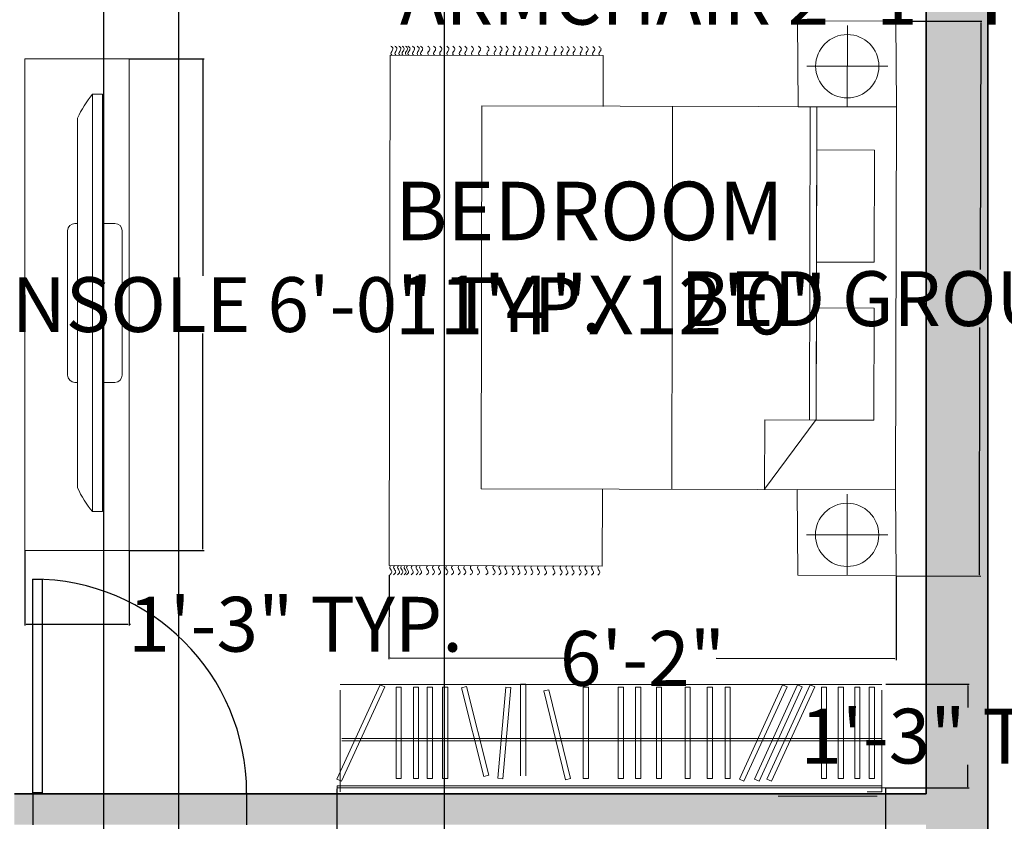
# Model space of a CAD drawing. Units: inches. Extents: x -4737294 to -4736756, y 1716389 to 1717040.
# Tile 23 of 25: x -4736996 to -4736853, y 1716845 to 1716962. Entities that reach past the tile are written whole.
import ezdxf

# ---------------------------------------------------------------- set-up
doc = ezdxf.new("R2010")
doc.units = ezdxf.units.IN
doc.header["$MEASUREMENT"] = 0
for name, color, linetype, lineweight in [('A-ANNO-DIMS', 2, 'Continuous', 18), ('A-AREA-IDEN', 250, 'Continuous', 18), ('A-WALL-PATT', 244, 'Continuous', 13), ('closet', 252, 'Continuous', 18), ('doors', 252, 'Continuous', 25), ('furniture', 250, 'Continuous', 18), ('walls', 252, 'Continuous', 35)]:
    doc.layers.add(name, color=color, linetype=linetype, lineweight=lineweight)
doc.styles.get("Standard").update_dxf_attribs({"font": 'arial.ttf'})
doc.dimstyles.get("Standard").update_dxf_attribs({"dimtxt": 8, "dimasz": 0.18, "dimexe": 0.18, "dimexo": 0.0625, "dimgap": 0.09, "dimtad": 0, "dimtih": 1, "dimtoh": 1, "dimzin": 0, "dimdsep": 46, "dimlunit": 3, "dimtxsty": 'Standard', "dimcen": 0.09, "dimadec": 0, "dimazin": 0, "dimtfac": 1, "dimtofl": 0, "dimtmove": 0, "dimatfit": 3, "dimfxl": 1, "dimtolj": 1, "dimtzin": 0, "dimarcsym": 0})

# ---------------------------------------------------------------- blocks, each defined once
blk = doc.blocks.new('*D22')
at = {"layer": 'A-ANNO-DIMS', "color": 0, "lineweight": -2, "transparency": 16777216}
for p, q in [((-4736855.08, 1717002.06), (-4736830.06, 1717002.06)), ((-4736830.24, 1717001.88), (-4736830.24, 1716736.22)), ((-4736830.24, 1716462.24), (-4736830.24, 1716727.91)), ((-4736855.08, 1716462.06), (-4736830.06, 1716462.06))]:
    blk.add_line(p, q, dxfattribs=at)
at = {"layer": 'A-ANNO-DIMS', "color": 0, "transparency": 16777216}
for points in [[(-4736830.27, 1717001.88), (-4736830.21, 1717001.88), (-4736830.24, 1717002.06)], [(-4736830.27, 1716462.24), (-4736830.21, 1716462.24), (-4736830.24, 1716462.06)]]:
    blk.add_solid(points, dxfattribs=at)
at = {"layer": 'Defpoints', "color": 0, "transparency": 16777216}
for p in [(-4736855.14, 1717002.06), (-4736830.24, 1717002.06), (-4736855.14, 1716462.06)]:
    blk.add_point(p, dxfattribs=at)
at = {"layer": 'A-ANNO-DIMS', "color": 0, "transparency": 16777216, "insert": (-4736830.24, 1716732.06), "char_height": 8, "attachment_point": 5}
blk.add_mtext("\\A1;45'", dxfattribs=at)
blk = doc.blocks.new('CARPET')
at = {"layer": 'furniture'}
for p, q in [((-51.53, -98.11), (-51.53, -55.12)), ((-51.53, -55.12), (-41.27, -55.12)), ((36, -55.12), (51.55, -55.12)), ((51.55, -55.12), (51.55, -98.11)), ((51.55, -98.11), (-51.53, -98.11))]:
    blk.add_line(p, q, dxfattribs=at)
for points, knots in [([(-53.37, -55.99), (-53.22, -55.8), (-52.9, -55.41), (-52.34, -55.8), (-51.89, -56.08), (-51.65, -55.91), (-51.53, -55.83)], [0, 0, 0, 0, 0.653278, 1.290138, 1.740457, 2.114451, 2.114451, 2.114451, 2.114451]), ([(53.37, -55.99), (53.22, -55.8), (52.9, -55.41), (52.34, -55.8), (51.89, -56.08), (51.65, -55.91), (51.53, -55.83)], [0, 0, 0, 0, 0.653278, 1.290138, 1.740457, 2.114451, 2.114451, 2.114451, 2.114451]), ([(-53.37, -57.26), (-53.22, -57.07), (-52.9, -56.67), (-52.34, -57.07), (-51.89, -57.35), (-51.65, -57.17), (-51.53, -57.1)], [0, 0, 0, 0, 0.653278, 1.290138, 1.740457, 2.114451, 2.114451, 2.114451, 2.114451]), ([(53.37, -57.26), (53.22, -57.07), (52.9, -56.67), (52.34, -57.07), (51.89, -57.35), (51.65, -57.17), (51.53, -57.1)], [0, 0, 0, 0, 0.653278, 1.290138, 1.740457, 2.114451, 2.114451, 2.114451, 2.114451]), ([(-53.37, -58.59), (-53.22, -58.4), (-52.9, -58.01), (-52.34, -58.4), (-51.89, -58.68), (-51.65, -58.5), (-51.53, -58.43)], [0, 0, 0, 0, 0.653278, 1.290138, 1.740457, 2.114451, 2.114451, 2.114451, 2.114451]), ([(-53.37, -59.78), (-53.22, -59.58), (-52.9, -59.19), (-52.34, -59.58), (-51.89, -59.86), (-51.65, -59.69), (-51.53, -59.61)], [0, 0, 0, 0, 0.653278, 1.290138, 1.740457, 2.114451, 2.114451, 2.114451, 2.114451]), ([(53.37, -58.59), (53.22, -58.4), (52.9, -58.01), (52.34, -58.4), (51.89, -58.68), (51.65, -58.5), (51.53, -58.43)], [0, 0, 0, 0, 0.653278, 1.290138, 1.740457, 2.114451, 2.114451, 2.114451, 2.114451]), ([(53.37, -59.78), (53.22, -59.58), (52.9, -59.19), (52.34, -59.58), (51.89, -59.86), (51.65, -59.69), (51.53, -59.61)], [0, 0, 0, 0, 0.653278, 1.290138, 1.740457, 2.114451, 2.114451, 2.114451, 2.114451]), ([(-53.37, -61.22), (-53.22, -61.02), (-52.9, -60.63), (-52.34, -61.02), (-51.89, -61.3), (-51.65, -61.13), (-51.53, -61.05)], [0, 0, 0, 0, 0.653278, 1.290138, 1.740457, 2.114451, 2.114451, 2.114451, 2.114451]), ([(53.37, -61.22), (53.22, -61.02), (52.9, -60.63), (52.34, -61.02), (51.89, -61.3), (51.65, -61.13), (51.53, -61.05)], [0, 0, 0, 0, 0.653278, 1.290138, 1.740457, 2.114451, 2.114451, 2.114451, 2.114451]), ([(-53.37, -62.44), (-53.22, -62.25), (-52.9, -61.86), (-52.34, -62.25), (-51.89, -62.53), (-51.65, -62.36), (-51.53, -62.28)], [0, 0, 0, 0, 0.653278, 1.290138, 1.740457, 2.114451, 2.114451, 2.114451, 2.114451]), ([(-53.37, -63.63), (-53.22, -63.43), (-52.9, -63.04), (-52.34, -63.43), (-51.89, -63.72), (-51.65, -63.54), (-51.53, -63.46)], [0, 0, 0, 0, 0.653278, 1.290138, 1.740457, 2.114451, 2.114451, 2.114451, 2.114451]), ([(53.37, -62.44), (53.22, -62.25), (52.9, -61.86), (52.34, -62.25), (51.89, -62.53), (51.65, -62.36), (51.53, -62.28)], [0, 0, 0, 0, 0.653278, 1.290138, 1.740457, 2.114451, 2.114451, 2.114451, 2.114451]), ([(53.37, -63.63), (53.22, -63.43), (52.9, -63.04), (52.34, -63.43), (51.89, -63.72), (51.65, -63.54), (51.53, -63.46)], [0, 0, 0, 0, 0.653278, 1.290138, 1.740457, 2.114451, 2.114451, 2.114451, 2.114451]), ([(-53.37, -65.07), (-53.22, -64.87), (-52.9, -64.48), (-52.34, -64.87), (-51.89, -65.15), (-51.65, -64.98), (-51.53, -64.9)], [0, 0, 0, 0, 0.653278, 1.290138, 1.740457, 2.114451, 2.114451, 2.114451, 2.114451]), ([(53.37, -65.07), (53.22, -64.87), (52.9, -64.48), (52.34, -64.87), (51.89, -65.15), (51.65, -64.98), (51.53, -64.9)], [0, 0, 0, 0, 0.653278, 1.290138, 1.740457, 2.114451, 2.114451, 2.114451, 2.114451]), ([(-53.37, -66.76), (-53.22, -66.56), (-52.9, -66.17), (-52.34, -66.56), (-51.89, -66.84), (-51.65, -66.67), (-51.53, -66.59)], [0, 0, 0, 0, 0.653278, 1.290138, 1.740457, 2.114451, 2.114451, 2.114451, 2.114451]), ([(53.37, -66.76), (53.22, -66.56), (52.9, -66.17), (52.34, -66.56), (51.89, -66.84), (51.65, -66.67), (51.53, -66.59)], [0, 0, 0, 0, 0.653278, 1.290138, 1.740457, 2.114451, 2.114451, 2.114451, 2.114451]), ([(-53.37, -68.2), (-53.22, -68), (-52.9, -67.61), (-52.34, -68), (-51.89, -68.28), (-51.65, -68.11), (-51.53, -68.03)], [0, 0, 0, 0, 0.653278, 1.290138, 1.740457, 2.114451, 2.114451, 2.114451, 2.114451]), ([(-53.37, -69.53), (-53.22, -69.33), (-52.9, -68.94), (-52.34, -69.33), (-51.89, -69.61), (-51.65, -69.44), (-51.53, -69.36)], [0, 0, 0, 0, 0.653278, 1.290138, 1.740457, 2.114451, 2.114451, 2.114451, 2.114451]), ([(53.37, -68.2), (53.22, -68), (52.9, -67.61), (52.34, -68), (51.89, -68.28), (51.65, -68.11), (51.53, -68.03)], [0, 0, 0, 0, 0.653278, 1.290138, 1.740457, 2.114451, 2.114451, 2.114451, 2.114451]), ([(53.37, -69.53), (53.22, -69.33), (52.9, -68.94), (52.34, -69.33), (51.89, -69.61), (51.65, -69.44), (51.53, -69.36)], [0, 0, 0, 0, 0.653278, 1.290138, 1.740457, 2.114451, 2.114451, 2.114451, 2.114451]), ([(-53.37, -70.79), (-53.22, -70.6), (-52.9, -70.21), (-52.34, -70.6), (-51.89, -70.88), (-51.65, -70.7), (-51.53, -70.63)], [0, 0, 0, 0, 0.653278, 1.290138, 1.740457, 2.114451, 2.114451, 2.114451, 2.114451]), ([(53.37, -70.79), (53.22, -70.6), (52.9, -70.21), (52.34, -70.6), (51.89, -70.88), (51.65, -70.7), (51.53, -70.63)], [0, 0, 0, 0, 0.653278, 1.290138, 1.740457, 2.114451, 2.114451, 2.114451, 2.114451]), ([(-53.37, -72.12), (-53.22, -71.93), (-52.9, -71.54), (-52.34, -71.93), (-51.89, -72.21), (-51.65, -72.04), (-51.53, -71.96)], [0, 0, 0, 0, 0.653278, 1.290138, 1.740457, 2.114451, 2.114451, 2.114451, 2.114451]), ([(-53.37, -73.31), (-53.22, -73.11), (-52.9, -72.72), (-52.34, -73.11), (-51.89, -73.4), (-51.65, -73.22), (-51.53, -73.14)], [0, 0, 0, 0, 0.653278, 1.290138, 1.740457, 2.114451, 2.114451, 2.114451, 2.114451]), ([(53.37, -72.12), (53.22, -71.93), (52.9, -71.54), (52.34, -71.93), (51.89, -72.21), (51.65, -72.04), (51.53, -71.96)], [0, 0, 0, 0, 0.653278, 1.290138, 1.740457, 2.114451, 2.114451, 2.114451, 2.114451]), ([(53.37, -73.31), (53.22, -73.11), (52.9, -72.72), (52.34, -73.11), (51.89, -73.4), (51.65, -73.22), (51.53, -73.14)], [0, 0, 0, 0, 0.653278, 1.290138, 1.740457, 2.114451, 2.114451, 2.114451, 2.114451]), ([(-53.37, -74.75), (-53.22, -74.55), (-52.9, -74.16), (-52.34, -74.55), (-51.89, -74.83), (-51.65, -74.66), (-51.53, -74.58)], [0, 0, 0, 0, 0.653278, 1.290138, 1.740457, 2.114451, 2.114451, 2.114451, 2.114451]), ([(53.37, -74.75), (53.22, -74.55), (52.9, -74.16), (52.34, -74.55), (51.89, -74.83), (51.65, -74.66), (51.53, -74.58)], [0, 0, 0, 0, 0.653278, 1.290138, 1.740457, 2.114451, 2.114451, 2.114451, 2.114451]), ([(-53.37, -75.98), (-53.22, -75.78), (-52.9, -75.39), (-52.34, -75.78), (-51.89, -76.06), (-51.65, -75.89), (-51.53, -75.81)], [0, 0, 0, 0, 0.653278, 1.290138, 1.740457, 2.114451, 2.114451, 2.114451, 2.114451]), ([(-53.37, -77.16), (-53.22, -76.96), (-52.9, -76.57), (-52.34, -76.96), (-51.89, -77.25), (-51.65, -77.07), (-51.53, -76.99)], [0, 0, 0, 0, 0.653278, 1.290138, 1.740457, 2.114451, 2.114451, 2.114451, 2.114451]), ([(53.37, -75.98), (53.22, -75.78), (52.9, -75.39), (52.34, -75.78), (51.89, -76.06), (51.65, -75.89), (51.53, -75.81)], [0, 0, 0, 0, 0.653278, 1.290138, 1.740457, 2.114451, 2.114451, 2.114451, 2.114451]), ([(53.37, -77.16), (53.22, -76.96), (52.9, -76.57), (52.34, -76.96), (51.89, -77.25), (51.65, -77.07), (51.53, -76.99)], [0, 0, 0, 0, 0.653278, 1.290138, 1.740457, 2.114451, 2.114451, 2.114451, 2.114451]), ([(-53.37, -78.6), (-53.22, -78.4), (-52.9, -78.01), (-52.34, -78.4), (-51.89, -78.68), (-51.65, -78.51), (-51.53, -78.43)], [0, 0, 0, 0, 0.653278, 1.290138, 1.740457, 2.114451, 2.114451, 2.114451, 2.114451]), ([(53.37, -78.6), (53.22, -78.4), (52.9, -78.01), (52.34, -78.4), (51.89, -78.68), (51.65, -78.51), (51.53, -78.43)], [0, 0, 0, 0, 0.653278, 1.290138, 1.740457, 2.114451, 2.114451, 2.114451, 2.114451]), ([(-53.37, -80.29), (-53.22, -80.09), (-52.9, -79.7), (-52.34, -80.09), (-51.89, -80.37), (-51.65, -80.2), (-51.53, -80.12)], [0, 0, 0, 0, 0.653278, 1.290138, 1.740457, 2.114451, 2.114451, 2.114451, 2.114451]), ([(-53.37, -81.73), (-53.22, -81.53), (-52.9, -81.14), (-52.34, -81.53), (-51.89, -81.81), (-51.65, -81.64), (-51.53, -81.56)], [0, 0, 0, 0, 0.653278, 1.290138, 1.740457, 2.114451, 2.114451, 2.114451, 2.114451]), ([(53.37, -80.29), (53.22, -80.09), (52.9, -79.7), (52.34, -80.09), (51.89, -80.37), (51.65, -80.2), (51.53, -80.12)], [0, 0, 0, 0, 0.653278, 1.290138, 1.740457, 2.114451, 2.114451, 2.114451, 2.114451]), ([(53.37, -81.73), (53.22, -81.53), (52.9, -81.14), (52.34, -81.53), (51.89, -81.81), (51.65, -81.64), (51.53, -81.56)], [0, 0, 0, 0, 0.653278, 1.290138, 1.740457, 2.114451, 2.114451, 2.114451, 2.114451]), ([(-53.37, -83.06), (-53.22, -82.86), (-52.9, -82.47), (-52.34, -82.86), (-51.89, -83.14), (-51.65, -82.97), (-51.53, -82.89)], [0, 0, 0, 0, 0.653278, 1.290138, 1.740457, 2.114451, 2.114451, 2.114451, 2.114451]), ([(53.37, -83.06), (53.22, -82.86), (52.9, -82.47), (52.34, -82.86), (51.89, -83.14), (51.65, -82.97), (51.53, -82.89)], [0, 0, 0, 0, 0.653278, 1.290138, 1.740457, 2.114451, 2.114451, 2.114451, 2.114451]), ([(-53.37, -84.18), (-53.22, -83.99), (-52.9, -83.6), (-52.34, -83.99), (-51.89, -84.27), (-51.65, -84.09), (-51.53, -84.02)], [0, 0, 0, 0, 0.653278, 1.290138, 1.740457, 2.114451, 2.114451, 2.114451, 2.114451]), ([(-53.37, -85.51), (-53.22, -85.32), (-52.9, -84.93), (-52.34, -85.32), (-51.89, -85.6), (-51.65, -85.42), (-51.53, -85.35)], [0, 0, 0, 0, 0.653278, 1.290138, 1.740457, 2.114451, 2.114451, 2.114451, 2.114451]), ([(53.37, -84.18), (53.22, -83.99), (52.9, -83.6), (52.34, -83.99), (51.89, -84.27), (51.65, -84.09), (51.53, -84.02)], [0, 0, 0, 0, 0.653278, 1.290138, 1.740457, 2.114451, 2.114451, 2.114451, 2.114451]), ([(53.37, -85.51), (53.22, -85.32), (52.9, -84.93), (52.34, -85.32), (51.89, -85.6), (51.65, -85.42), (51.53, -85.35)], [0, 0, 0, 0, 0.653278, 1.290138, 1.740457, 2.114451, 2.114451, 2.114451, 2.114451]), ([(-53.37, -86.7), (-53.22, -86.5), (-52.9, -86.11), (-52.34, -86.5), (-51.89, -86.78), (-51.65, -86.61), (-51.53, -86.53)], [0, 0, 0, 0, 0.653278, 1.290138, 1.740457, 2.114451, 2.114451, 2.114451, 2.114451]), ([(53.37, -86.7), (53.22, -86.5), (52.9, -86.11), (52.34, -86.5), (51.89, -86.78), (51.65, -86.61), (51.53, -86.53)], [0, 0, 0, 0, 0.653278, 1.290138, 1.740457, 2.114451, 2.114451, 2.114451, 2.114451]), ([(-53.37, -88.14), (-53.22, -87.94), (-52.9, -87.55), (-52.34, -87.94), (-51.89, -88.22), (-51.65, -88.05), (-51.53, -87.97)], [0, 0, 0, 0, 0.653278, 1.290138, 1.740457, 2.114451, 2.114451, 2.114451, 2.114451]), ([(-53.37, -89.36), (-53.22, -89.17), (-52.9, -88.78), (-52.34, -89.17), (-51.89, -89.45), (-51.65, -89.28), (-51.53, -89.2)], [0, 0, 0, 0, 0.653278, 1.290138, 1.740457, 2.114451, 2.114451, 2.114451, 2.114451]), ([(53.37, -88.14), (53.22, -87.94), (52.9, -87.55), (52.34, -87.94), (51.89, -88.22), (51.65, -88.05), (51.53, -87.97)], [0, 0, 0, 0, 0.653278, 1.290138, 1.740457, 2.114451, 2.114451, 2.114451, 2.114451]), ([(53.37, -89.36), (53.22, -89.17), (52.9, -88.78), (52.34, -89.17), (51.89, -89.45), (51.65, -89.28), (51.53, -89.2)], [0, 0, 0, 0, 0.653278, 1.290138, 1.740457, 2.114451, 2.114451, 2.114451, 2.114451]), ([(-53.37, -90.55), (-53.22, -90.35), (-52.9, -89.96), (-52.34, -90.35), (-51.89, -90.64), (-51.65, -90.46), (-51.53, -90.38)], [0, 0, 0, 0, 0.653278, 1.290138, 1.740457, 2.114451, 2.114451, 2.114451, 2.114451]), ([(53.37, -90.55), (53.22, -90.35), (52.9, -89.96), (52.34, -90.35), (51.9, -90.63), (51.66, -90.47), (51.55, -90.4)], [0, 0, 0, 0, 0.653278, 1.290138, 1.740457, 2.0926, 2.0926, 2.0926, 2.0926]), ([(-53.37, -91.99), (-53.22, -91.79), (-52.9, -91.4), (-52.34, -91.79), (-51.89, -92.07), (-51.65, -91.9), (-51.53, -91.82)], [0, 0, 0, 0, 0.653278, 1.290138, 1.740457, 2.114451, 2.114451, 2.114451, 2.114451]), ([(-53.37, -92.69), (-53.22, -92.48), (-52.9, -92.08), (-52.35, -92.49), (-51.89, -92.77), (-51.65, -92.6), (-51.53, -92.52)], [0, 0, 0, 0, 0.663904, 1.307406, 1.757725, 2.131719, 2.131719, 2.131719, 2.131719]), ([(-53.37, -93.61), (-53.22, -93.42), (-52.9, -93.03), (-52.34, -93.42), (-51.89, -93.7), (-51.65, -93.52), (-51.53, -93.45)], [0, 0, 0, 0, 0.653278, 1.290138, 1.740457, 2.114451, 2.114451, 2.114451, 2.114451]), ([(53.37, -91.99), (53.22, -91.79), (52.9, -91.4), (52.34, -91.79), (51.9, -92.07), (51.66, -91.91), (51.55, -91.83)], [0, 0, 0, 0, 0.653278, 1.290138, 1.740457, 2.0926, 2.0926, 2.0926, 2.0926]), ([(53.37, -92.69), (53.22, -92.49), (52.9, -92.09), (52.34, -92.49), (51.9, -92.77), (51.66, -92.61), (51.55, -92.53)], [0, 0, 0, 0, 0.656792, 1.295826, 1.746145, 2.098292, 2.098292, 2.098292, 2.098292]), ([(53.37, -93.66), (53.22, -93.46), (52.9, -93.07), (52.34, -93.46), (51.9, -93.74), (51.66, -93.58), (51.55, -93.5)], [0, 0, 0, 0, 0.653278, 1.290138, 1.740457, 2.0926, 2.0926, 2.0926, 2.0926]), ([(-53.37, -94.55), (-53.22, -94.35), (-52.9, -93.96), (-52.34, -94.35), (-51.89, -94.63), (-51.65, -94.46), (-51.53, -94.38)], [0, 0, 0, 0, 0.653278, 1.290138, 1.740457, 2.114451, 2.114451, 2.114451, 2.114451]), ([(-53.37, -95.05), (-53.22, -94.85), (-52.9, -94.46), (-52.34, -94.85), (-51.89, -95.14), (-51.65, -94.96), (-51.53, -94.88)], [0, 0, 0, 0, 0.653278, 1.290138, 1.740457, 2.114451, 2.114451, 2.114451, 2.114451]), ([(-53.37, -95.73), (-53.22, -95.54), (-52.9, -95.15), (-52.34, -95.54), (-51.89, -95.82), (-51.65, -95.65), (-51.53, -95.57)], [0, 0, 0, 0, 0.653278, 1.290138, 1.740457, 2.114451, 2.114451, 2.114451, 2.114451]), ([(53.37, -95.78), (53.22, -95.58), (52.9, -95.19), (52.34, -95.58), (51.89, -95.86), (51.65, -95.69), (51.53, -95.61)], [0, 0, 0, 0, 0.653278, 1.290138, 1.740457, 2.114451, 2.114451, 2.114451, 2.114451]), ([(53.37, -94.59), (53.22, -94.4), (52.9, -94.01), (52.34, -94.4), (51.9, -94.68), (51.66, -94.51), (51.55, -94.44)], [0, 0, 0, 0, 0.653278, 1.290138, 1.740457, 2.0926, 2.0926, 2.0926, 2.0926]), ([(53.37, -95.1), (53.22, -94.9), (52.9, -94.51), (52.34, -94.9), (51.9, -95.18), (51.66, -95.02), (51.55, -94.94)], [0, 0, 0, 0, 0.653278, 1.290138, 1.740457, 2.0926, 2.0926, 2.0926, 2.0926]), ([(-53.37, -96.38), (-53.22, -96.18), (-52.9, -95.79), (-52.34, -96.18), (-51.89, -96.47), (-51.65, -96.29), (-51.53, -96.21)], [0, 0, 0, 0, 0.653278, 1.290138, 1.740457, 2.114451, 2.114451, 2.114451, 2.114451]), ([(-53.37, -97.17), (-53.22, -96.98), (-52.9, -96.59), (-52.34, -96.98), (-51.89, -97.26), (-51.65, -97.08), (-51.53, -97.01)], [0, 0, 0, 0, 0.653278, 1.290138, 1.740457, 2.114451, 2.114451, 2.114451, 2.114451]), ([(53.37, -96.43), (53.22, -96.23), (52.9, -95.84), (52.34, -96.23), (51.89, -96.51), (51.65, -96.34), (51.53, -96.26)], [0, 0, 0, 0, 0.653278, 1.290138, 1.740457, 2.114451, 2.114451, 2.114451, 2.114451]), ([(53.37, -97.22), (53.22, -97.02), (52.9, -96.63), (52.34, -97.02), (51.89, -97.3), (51.65, -97.13), (51.53, -97.05)], [0, 0, 0, 0, 0.653278, 1.290138, 1.740457, 2.114451, 2.114451, 2.114451, 2.114451]), ([(-53.37, -97.99), (-53.22, -97.79), (-52.9, -97.4), (-52.34, -97.79), (-51.89, -98.08), (-51.65, -97.9), (-51.53, -97.82)], [0, 0, 0, 0, 0.653278, 1.290138, 1.740457, 2.114451, 2.114451, 2.114451, 2.114451]), ([(53.37, -97.99), (53.22, -97.79), (52.9, -97.4), (52.34, -97.79), (51.89, -98.08), (51.65, -97.9), (51.53, -97.82)], [0, 0, 0, 0, 0.653278, 1.290138, 1.740457, 2.114451, 2.114451, 2.114451, 2.114451])]:
    blk.add_open_spline(points, degree=3, knots=knots, dxfattribs=at)
blk = doc.blocks.new('A$C58D270C6')
at = {"layer": 'furniture'}
for p, q in [((9.09, 124.13), (9.09, 108.87)), ((1.46, 116.5), (16.73, 116.5)), ((14.97, 94.84), (24.62, 107.92)), ((24.62, 94.93), (24.62, 107.92)), ((42.08, 108), (42.08, 36)), ((14.97, 94.93), (24.62, 94.93)), ((14.97, 94.84), (14.97, 36)), ((16.22, 94.93), (16.22, 36)), ((9.25, 36), (9.25, 20.74)), ((1.62, 28.37), (16.88, 28.37))]:
    blk.add_line(p, q, dxfattribs=at)
for points in [[(18.5, 108), (18.34, 124.13), (-0.16, 124.13), (0, 108)], [(0, 108), (77.91, 108), (77.91, 36), (0, 36)], [(4.09, 94.93), (14.97, 94.93), (14.97, 73.83), (4.09, 73.83)], [(4.09, 65.23), (14.97, 65.23), (14.97, 44.13), (4.09, 44.13)], [(18.65, 19.87), (18.5, 36), (0, 36), (0.16, 19.87)]]:
    blk.add_lwpolyline(points, close=True, dxfattribs=at)
for centre in [(9.09, 116.5), (9.25, 28.37)]:
    blk.add_circle(centre, 5.95, dxfattribs=at)
at = {"layer": 'furniture', "xscale": 0.9312884925094044, "yscale": 0.9312884925094044, "zscale": 0.9312884925094044, "rotation": 90}
blk.add_blockref('CARPET', (3.79, 74.47), dxfattribs=at)
blk = doc.blocks.new('closet')
at = {"layer": 'closet'}
for p, q in [((-0.71, -5.58), (5.59, 8.19)), ((-0.23, 7.39), (-0.23, -6.57)), ((6.27, 7.88), (-0.04, -5.89)), ((5.59, 8.19), (6.27, 7.88)), ((7.92, 7.84), (8.68, 7.84)), ((7.92, 7.84), (7.92, -5.51)), ((8.68, 7.84), (8.68, -5.51)), ((10.44, 7.84), (11.2, 7.84)), ((10.44, 7.84), (10.44, -5.51)), ((11.2, 7.84), (11.2, -5.51)), ((12.45, 7.84), (13.21, 7.84)), ((12.45, 7.84), (12.45, -5.51)), ((13.21, 7.84), (13.21, -5.51)), ((14.71, 7.84), (15.47, 7.84)), ((14.71, 7.84), (14.71, -5.51)), ((15.47, 7.84), (15.47, -5.51)), ((17.44, 7.75), (18.17, 7.93)), ((17.44, 7.75), (20.73, -5.2)), ((18.17, 7.93), (21.46, -5.01)), ((23.92, 7.84), (22.75, -5.46)), ((24.67, 7.78), (23.51, -5.53)), ((23.92, 7.84), (24.67, 7.78)), ((26.09, 8.25), (26.09, -5.1)), ((26.84, 8.25), (26.84, -5.1)), ((29.49, 7.29), (32.64, -5.69)), ((30.22, 7.46), (33.37, -5.51)), ((35.23, 7.84), (35.23, -5.51)), ((35.99, 7.84), (35.99, -5.51)), ((40.33, 7.84), (40.33, -5.51)), ((41.08, 7.84), (41.08, -5.51)), ((42.85, 7.84), (42.85, -5.51)), ((43.61, 7.84), (43.61, -5.51)), ((45.9, 7.84), (45.9, -5.51)), ((46.65, 7.84), (46.65, -5.51)), ((50.07, 7.84), (50.07, -5.51)), ((50.82, 7.84), (50.82, -5.51)), ((53.32, 7.84), (53.32, -5.51)), ((54.08, 7.84), (54.08, -5.51)), ((55.9, 7.84), (55.9, -5.51)), ((56.65, 7.84), (56.65, -5.51)), ((57.99, -5.58), (64.3, 8.19)), ((64.97, 7.88), (58.67, -5.89)), ((60.19, -5.58), (66.49, 8.19)), ((67.17, 7.88), (60.87, -5.89)), ((62, -5.58), (68.3, 8.19)), ((68.98, 7.88), (62.67, -5.89)), ((69.96, 7.84), (69.96, -5.51)), ((70.72, 7.84), (70.72, -5.51)), ((72.43, 7.84), (72.43, -5.51)), ((73.19, 7.84), (73.19, -5.51)), ((74.82, 7.84), (74.82, -5.51)), ((75.57, 7.84), (75.57, -5.51)), ((76.94, 7.84), (76.94, -5.51)), ((77.69, 7.84), (77.69, -5.51)), ((56.23, 0.33), (0, 0.33)), ((56.2, 0), (0, 0)), ((56.2, 0), (78.76, 0)), ((56.23, 0.33), (78.76, 0.33)), ((-0.04, -5.89), (-0.71, -5.58)), ((21.46, -5.01), (20.73, -5.2)), ((23.51, -5.53), (22.75, -5.46)), ((33.37, -5.51), (32.64, -5.69)), ((35.99, -5.51), (35.23, -5.51)), ((41.08, -5.51), (40.33, -5.51)), ((43.61, -5.51), (42.85, -5.51)), ((46.65, -5.51), (45.9, -5.51)), ((50.82, -5.51), (50.07, -5.51)), ((54.08, -5.51), (53.32, -5.51)), ((56.65, -5.51), (55.9, -5.51)), ((58.67, -5.89), (57.99, -5.58)), ((60.87, -5.89), (60.19, -5.58)), ((62.67, -5.89), (62, -5.58)), ((70.72, -5.51), (69.96, -5.51)), ((73.19, -5.51), (72.43, -5.51)), ((75.57, -5.51), (74.82, -5.51)), ((77.69, -5.51), (76.94, -5.51))]:
    blk.add_line(p, q, dxfattribs=at)
blk = doc.blocks.new('rotated closet')
at = {"layer": 'closet'}
for p, q in [((26.32, 0.86), (27.07, 0.86)), ((29.72, -0.11), (30.45, 0.07)), ((35.46, 0.45), (36.22, 0.45)), ((40.56, 0.45), (41.31, 0.45)), ((43.08, 0.45), (43.84, 0.45)), ((46.13, 0.45), (46.88, 0.45)), ((50.3, 0.45), (51.05, 0.45)), ((53.56, 0.45), (54.31, 0.45)), ((56.13, 0.45), (56.88, 0.45)), ((64.53, 0.8), (65.2, 0.49)), ((66.72, 0.8), (67.4, 0.49)), ((68.53, 0.8), (69.21, 0.49)), ((70.19, 0.45), (70.95, 0.45)), ((72.66, 0.45), (73.42, 0.45)), ((75.05, 0.45), (75.81, 0.45)), ((77.17, 0.45), (77.92, 0.45)), ((78.99, 0), (78.99, -13.96)), ((8.91, -12.91), (8.15, -12.91)), ((11.43, -12.91), (10.67, -12.91)), ((13.44, -12.91), (12.68, -12.91)), ((15.7, -12.91), (14.94, -12.91)), ((-0.46, -14.27), (79.54, -14.27)), ((0, -13.96), (78.99, -13.96))]:
    blk.add_line(p, q, dxfattribs=at)
blk.add_blockref('closet', (0.23, -7.39), dxfattribs=at)
blk = doc.blocks.new('*U20')
for p, q in [((0, 0), (0, -6)), ((40, 0), (40, -6))]:
    blk.add_line(p, q)
blk.add_lwpolyline([(0, 0), (0, 40), (1.75, 40), (1.75, 0)], close=True)
blk.add_arc((0, 0), 40, 0, 90)
blk = doc.blocks.new('PLASMA-LARGE')
at = {"layer": 'furniture'}
for p, q in [((-7.256, 0), (7.256, 0)), ((-8, -1), (-8, -0.744)), ((8, -1), (8, -0.744)), ((-18.608, -1), (18.608, -1)), ((-21, -2.5), (21, -2.5)), ((-21, -2.5), (-21, -3.5)), ((21, -2.5), (21, -3.5)), ((-21, -3.5), (21, -3.5)), ((-8, -3.5), (-8, -4.756)), ((8, -3.5), (8, -4.756)), ((-7.256, -5.5), (7.256, -5.5))]:
    blk.add_line(p, q, dxfattribs=at)
for centre, radius, start, end in [((-7.256, -0.744), 0.744, 90, 180), ((7.256, -0.744), 0.744, 0, 90), ((-13.972, -11.05), 11.068, 114.76019, 129.41749), ((13.972, -11.05), 11.068, 50.58251, 65.23981), ((-7.256, -4.756), 0.744, 180, 270), ((7.256, -4.756), 0.744, 270, 0)]:
    blk.add_arc(centre, radius, start, end, dxfattribs=at)
blk = doc.blocks.new('TV-CONSOLE-BEDROOM')
for p, q in [((15.21, 71.77), (0, 71.77)), ((0, 71.77), (0, 0)), ((15.21, 0), (15.21, 71.77)), ((0, 0), (15.21, 0))]:
    blk.add_line(p, q)
at = {"xscale": 1.450199298177205, "yscale": 1.450199298177205, "zscale": 1.450199298177205, "rotation": 90}
blk.add_blockref('PLASMA-LARGE', (6.22, 36.13), dxfattribs=at)
blk = doc.blocks.new('*D27')
at = {"layer": 'A-ANNO-DIMS', "color": 0, "lineweight": -2, "transparency": 16777216}
for p, q in [((-4736969.31, 1716969), (-4736969.31, 1716965.16)), ((-4736944.45, 1716969), (-4736944.45, 1716965.16)), ((-4736969.13, 1716965.34), (-4736944.63, 1716965.34)), ((-4736944.45, 1716965.34), (-4736944.27, 1716965.34))]:
    blk.add_line(p, q, dxfattribs=at)
at = {"layer": 'A-ANNO-DIMS', "color": 0, "transparency": 16777216}
for points in [[(-4736969.13, 1716965.37), (-4736969.13, 1716965.31), (-4736969.31, 1716965.34)], [(-4736944.63, 1716965.37), (-4736944.63, 1716965.31), (-4736944.45, 1716965.34)]]:
    blk.add_solid(points, dxfattribs=at)
at = {"layer": 'Defpoints', "color": 0, "transparency": 16777216}
for p in [(-4736969.31, 1716969.06), (-4736944.45, 1716969.06), (-4736944.45, 1716965.34)]:
    blk.add_point(p, dxfattribs=at)
at = {"layer": 'A-ANNO-DIMS', "color": 0, "transparency": 16777216, "insert": (-4736888.21, 1716965.34), "char_height": 8, "attachment_point": 5}
blk.add_mtext('\\A1;ARMCHAIR 2\'-1" TYP.', dxfattribs=at)
blk = doc.blocks.new('*D35')
at = {"layer": 'A-ANNO-DIMS', "color": 0, "lineweight": -2, "transparency": 16777216}
for p, q in [((-4736868.27, 1716961.85), (-4736856.01, 1716961.83)), ((-4736856.19, 1716961.65), (-4736856.27, 1716925.58)), ((-4736856.37, 1716881.05), (-4736856.29, 1716917.12)), ((-4736868.45, 1716880.9), (-4736856.19, 1716880.87))]:
    blk.add_line(p, q, dxfattribs=at)
at = {"layer": 'A-ANNO-DIMS', "color": 0, "transparency": 16777216}
for points in [[(-4736856.22, 1716961.65), (-4736856.16, 1716961.65), (-4736856.19, 1716961.83)], [(-4736856.4, 1716881.05), (-4736856.34, 1716881.05), (-4736856.37, 1716880.87)]]:
    blk.add_solid(points, dxfattribs=at)
at = {"layer": 'Defpoints', "color": 0, "transparency": 16777216}
for p in [(-4736868.33, 1716961.85), (-4736868.51, 1716880.9), (-4736856.37, 1716880.87)]:
    blk.add_point(p, dxfattribs=at)
at = {"layer": 'A-ANNO-DIMS', "color": 0, "transparency": 16777216, "insert": (-4736856.28, 1716921.35), "char_height": 8, "attachment_point": 5}
blk.add_mtext('\\A1;BED GROUP 6\'-9"', dxfattribs=at)
blk = doc.blocks.new('*D36')
at = {"layer": 'A-ANNO-DIMS', "color": 0, "lineweight": -2, "transparency": 16777216}
for p, q in [((-4736942.48, 1716881), (-4736942.51, 1716868.74)), ((-4736868.51, 1716880.84), (-4736868.54, 1716868.58)), ((-4736942.33, 1716868.92), (-4736916.27, 1716868.86)), ((-4736868.71, 1716868.76), (-4736894.78, 1716868.81))]:
    blk.add_line(p, q, dxfattribs=at)
at = {"layer": 'A-ANNO-DIMS', "color": 0, "transparency": 16777216}
for points in [[(-4736942.33, 1716868.95), (-4736942.33, 1716868.89), (-4736942.51, 1716868.92)], [(-4736868.71, 1716868.79), (-4736868.71, 1716868.73), (-4736868.53, 1716868.76)]]:
    blk.add_solid(points, dxfattribs=at)
at = {"layer": 'Defpoints', "color": 0, "transparency": 16777216}
for p in [(-4736942.48, 1716881.06), (-4736868.51, 1716880.9), (-4736942.51, 1716868.92)]:
    blk.add_point(p, dxfattribs=at)
at = {"layer": 'A-ANNO-DIMS', "color": 0, "transparency": 16777216, "insert": (-4736905.52, 1716868.84), "char_height": 8, "attachment_point": 5}
blk.add_mtext('\\A1;6\'-2"', dxfattribs=at)
blk = doc.blocks.new('*D43')
at = {"layer": 'A-ANNO-DIMS', "color": 0, "lineweight": -2, "transparency": 16777216}
for p, q in [((-4736980.34, 1716956.36), (-4736969.46, 1716956.36)), ((-4736969.64, 1716956.18), (-4736969.64, 1716924.7)), ((-4736969.64, 1716884.77), (-4736969.64, 1716916.25)), ((-4736980.34, 1716884.59), (-4736969.46, 1716884.59))]:
    blk.add_line(p, q, dxfattribs=at)
at = {"layer": 'A-ANNO-DIMS', "color": 0, "transparency": 16777216}
for points in [[(-4736969.67, 1716956.18), (-4736969.61, 1716956.18), (-4736969.64, 1716956.36)], [(-4736969.67, 1716884.77), (-4736969.61, 1716884.77), (-4736969.64, 1716884.59)]]:
    blk.add_solid(points, dxfattribs=at)
at = {"layer": 'Defpoints', "color": 0, "transparency": 16777216}
for p in [(-4736980.4, 1716956.36), (-4736969.64, 1716956.36), (-4736980.4, 1716884.59)]:
    blk.add_point(p, dxfattribs=at)
at = {"layer": 'A-ANNO-DIMS', "color": 0, "transparency": 16777216, "insert": (-4736969.64, 1716920.48), "char_height": 8, "attachment_point": 5}
blk.add_mtext('\\A1;TV CONSOLE 6\'-0" TYP.', dxfattribs=at)
blk = doc.blocks.new('*D44')
at = {"layer": 'A-ANNO-DIMS', "color": 0, "lineweight": -2, "transparency": 16777216}
for p, q in [((-4736995.62, 1716884.53), (-4736995.62, 1716873.65)), ((-4736980.4, 1716884.53), (-4736980.4, 1716873.65)), ((-4736995.44, 1716873.83), (-4736980.58, 1716873.83)), ((-4736980.4, 1716873.83), (-4736980.22, 1716873.83))]:
    blk.add_line(p, q, dxfattribs=at)
at = {"layer": 'A-ANNO-DIMS', "color": 0, "transparency": 16777216}
for points in [[(-4736995.44, 1716873.86), (-4736995.44, 1716873.8), (-4736995.62, 1716873.83)], [(-4736980.58, 1716873.86), (-4736980.58, 1716873.8), (-4736980.4, 1716873.83)]]:
    blk.add_solid(points, dxfattribs=at)
at = {"layer": 'Defpoints', "color": 0, "transparency": 16777216}
for p in [(-4736995.62, 1716884.59), (-4736980.4, 1716884.59), (-4736980.4, 1716873.83)]:
    blk.add_point(p, dxfattribs=at)
at = {"layer": 'A-ANNO-DIMS', "color": 0, "transparency": 16777216, "insert": (-4736956.13, 1716873.83), "char_height": 8, "attachment_point": 5}
blk.add_mtext('\\A1;1\'-3" TYP.', dxfattribs=at)
blk = doc.blocks.new('*D47')
at = {"layer": 'A-ANNO-DIMS', "color": 0, "lineweight": -2, "transparency": 16777216}
for p, q in [((-4736950.1, 1716849.87), (-4736950.1, 1716837.75)), ((-4736870.07, 1716849.87), (-4736870.07, 1716837.75)), ((-4736949.92, 1716837.93), (-4736870.25, 1716837.93)), ((-4736870.07, 1716837.93), (-4736869.89, 1716837.93))]:
    blk.add_line(p, q, dxfattribs=at)
at = {"layer": 'A-ANNO-DIMS', "color": 0, "transparency": 16777216}
for points in [[(-4736949.92, 1716837.96), (-4736949.92, 1716837.9), (-4736950.1, 1716837.93)], [(-4736870.25, 1716837.96), (-4736870.25, 1716837.9), (-4736870.07, 1716837.93)]]:
    blk.add_solid(points, dxfattribs=at)
at = {"layer": 'Defpoints', "color": 0, "transparency": 16777216}
for p in [(-4736950.1, 1716849.93), (-4736870.07, 1716849.93), (-4736870.07, 1716837.93)]:
    blk.add_point(p, dxfattribs=at)
at = {"layer": 'A-ANNO-DIMS', "color": 0, "transparency": 16777216, "insert": (-4736810.8, 1716837.93), "char_height": 8, "attachment_point": 5}
blk.add_mtext('\\A1;WARDROBE 6\'-8" TYP.', dxfattribs=at)
blk = doc.blocks.new('*D48')
at = {"layer": 'A-ANNO-DIMS', "color": 0, "lineweight": -2, "transparency": 16777216}
for p, q in [((-4736870.01, 1716865.07), (-4736857.89, 1716865.07)), ((-4736858.07, 1716864.89), (-4736858.07, 1716861.68)), ((-4736858.07, 1716850.11), (-4736858.07, 1716853.32)), ((-4736870.01, 1716849.93), (-4736857.89, 1716849.93))]:
    blk.add_line(p, q, dxfattribs=at)
at = {"layer": 'A-ANNO-DIMS', "color": 0, "transparency": 16777216}
for points in [[(-4736858.1, 1716864.89), (-4736858.04, 1716864.89), (-4736858.07, 1716865.07)], [(-4736858.1, 1716850.11), (-4736858.04, 1716850.11), (-4736858.07, 1716849.93)]]:
    blk.add_solid(points, dxfattribs=at)
at = {"layer": 'Defpoints', "color": 0, "transparency": 16777216}
for p in [(-4736870.07, 1716865.07), (-4736858.07, 1716865.07), (-4736870.07, 1716849.93)]:
    blk.add_point(p, dxfattribs=at)
at = {"layer": 'A-ANNO-DIMS', "color": 0, "transparency": 16777216, "insert": (-4736858.07, 1716857.5), "char_height": 8, "attachment_point": 5}
blk.add_mtext('\\A1;1\'-3" TYP.', dxfattribs=at)
blk = doc.blocks.new('*D65')
at = {"layer": 'A-ANNO-DIMS', "color": 0, "lineweight": -2, "transparency": 16777216}
for p, q in [((-4737007.1, 1716596.13), (-4737007.1, 1717035.24)), ((-4736984.09, 1716596.13), (-4736984.09, 1717035.24)), ((-4737006.92, 1717035.06), (-4736984.27, 1717035.06)), ((-4736984.09, 1717035.06), (-4736983.91, 1717035.06))]:
    blk.add_line(p, q, dxfattribs=at)
at = {"layer": 'A-ANNO-DIMS', "color": 0, "transparency": 16777216}
for points in [[(-4737006.92, 1717035.09), (-4737006.92, 1717035.03), (-4737007.1, 1717035.06)], [(-4736984.27, 1717035.09), (-4736984.27, 1717035.03), (-4736984.09, 1717035.06)]]:
    blk.add_solid(points, dxfattribs=at)
at = {"layer": 'Defpoints', "color": 0, "transparency": 16777216}
for p in [(-4736984.09, 1717035.06), (-4737007.1, 1716596.06), (-4736984.09, 1716596.06)]:
    blk.add_point(p, dxfattribs=at)
at = {"layer": 'A-ANNO-DIMS', "color": 0, "transparency": 16777216, "insert": (-4736970.46, 1717035.06), "char_height": 8, "attachment_point": 5}
blk.add_mtext('\\A1;1\'-11"', dxfattribs=at)
blk = doc.blocks.new('*D66')
at = {"layer": 'A-ANNO-DIMS', "color": 0, "lineweight": -2, "transparency": 16777216}
for p, q in [((-4736973.14, 1716668.63), (-4736973.14, 1717035.24)), ((-4736934.39, 1716668.63), (-4736934.39, 1717035.24)), ((-4736972.96, 1717035.06), (-4736964.49, 1717035.06)), ((-4736934.57, 1717035.06), (-4736943.05, 1717035.06))]:
    blk.add_line(p, q, dxfattribs=at)
at = {"layer": 'A-ANNO-DIMS', "color": 0, "transparency": 16777216}
for points in [[(-4736972.96, 1717035.09), (-4736972.96, 1717035.03), (-4736973.14, 1717035.06)], [(-4736934.57, 1717035.09), (-4736934.57, 1717035.03), (-4736934.39, 1717035.06)]]:
    blk.add_solid(points, dxfattribs=at)
at = {"layer": 'Defpoints', "color": 0, "transparency": 16777216}
for p in [(-4736934.39, 1717035.06), (-4736973.14, 1716668.56), (-4736934.39, 1716668.56)]:
    blk.add_point(p, dxfattribs=at)
at = {"layer": 'A-ANNO-DIMS', "color": 0, "transparency": 16777216, "insert": (-4736953.77, 1717035.06), "char_height": 8, "attachment_point": 5}
blk.add_mtext('\\A1;3\'-3"', dxfattribs=at)

msp = doc.modelspace()

# ---------------------------------------------------------------- hatches: boundary and pattern name
at = {"layer": 'A-WALL-PATT'}
h = msp.add_hatch(color=256, dxfattribs=at)
h.dxf.hatch_style = 1
h.paths.add_polyline_path([(-4737206.144, 1716844.565), (-4737110.144, 1716844.565), (-4737110.144, 1716823.907), (-4737105.644, 1716823.907), (-4737105.644, 1716844.565), (-4737098.44, 1716844.565), (-4737098.44, 1716849.065), (-4737206.144, 1716849.065), (-4737206.144, 1716993.065), (-4736864.144, 1716993.065), (-4736864.144, 1716849.065), (-4736963.275, 1716849.065), (-4736994.446, 1716849.065), (-4736997.144, 1716849.065), (-4736997.144, 1716844.565), (-4736864.144, 1716844.565), (-4736864.144, 1716668.565), (-4736934.391, 1716668.565), (-4736934.391, 1716664.065), (-4736864.144, 1716664.065), (-4736864.144, 1716462.065), (-4736855.144, 1716462.065), (-4736855.144, 1717002.065), (-4737215.144, 1717002.065), (-4737215.144, 1716462.065), (-4737206.144, 1716462.065), (-4737206.144, 1716659.065), (-4737062.144, 1716659.065), (-4737062.144, 1716647.493), (-4737057.644, 1716647.493), (-4737057.644, 1716796.565), (-4737071.812, 1716796.565), (-4737071.812, 1716792.065), (-4737070.805, 1716792.065), (-4737062.144, 1716792.065), (-4737062.144, 1716668.065), (-4737206.144, 1716668.065), (-4737206.144, 1716792.065), (-4737093.784, 1716792.065), (-4737093.784, 1716796.565), (-4737206.144, 1716796.565)])
h = msp.add_hatch(color=256, dxfattribs=at)
h.dxf.hatch_style = 1
h.paths.add_polyline_path([(-4737057.644, 1716600.884), (-4737062.144, 1716600.884), (-4737062.144, 1716534.565), (-4736933.144, 1716534.565), (-4736933.144, 1716462.065), (-4736924.144, 1716462.065), (-4736924.144, 1716543.565), (-4736973.144, 1716543.565), (-4736973.144, 1716668.565), (-4736977.644, 1716668.565), (-4736977.644, 1716543.565), (-4737057.644, 1716543.565), (-4737057.644, 1716591.565), (-4737007.073, 1716591.565), (-4737007.073, 1716596.065), (-4737057.644, 1716596.065)])
h.paths.add_polyline_path([(-4736962.872, 1716471.065), (-4737062.144, 1716471.065), (-4737062.144, 1716462.065), (-4736962.872, 1716462.065)], flags=17)
h.paths.add_polyline_path([(-4737161.883, 1716716.26), (-4737096.689, 1716716.26), (-4737096.689, 1716729.349), (-4737161.883, 1716729.349)], flags=9)
h.paths.add_polyline_path([(-4737161.912, 1716729.958), (-4737095.809, 1716729.958), (-4737095.809, 1716743.222), (-4737161.912, 1716743.222)], flags=9)
h.paths.add_polyline_path([(-4736943.842, 1716913.818), (-4736878.647, 1716913.818), (-4736878.647, 1716926.907), (-4736943.842, 1716926.907)], flags=9)
h.paths.add_polyline_path([(-4736943.871, 1716927.516), (-4736877.767, 1716927.516), (-4736877.767, 1716940.78), (-4736943.871, 1716940.78)], flags=9)
h = msp.add_hatch(color=256, dxfattribs=at)
h.dxf.hatch_style = 1
h.paths.add_polyline_path([(-4736994.446, 1716849.065), (-4736997.144, 1716849.065), (-4736997.144, 1716844.565), (-4736994.446, 1716844.565)])
h.paths.add_polyline_path([(-4737023.821, 1716917.161), (-4737023.821, 1716880.778), (-4737014.648, 1716880.778), (-4737014.648, 1716917.161)], flags=9)
h.paths.add_polyline_path([(-4737014.221, 1716917.181), (-4737014.221, 1716884.798), (-4737004.926, 1716884.798), (-4737004.926, 1716917.181)], flags=9)

# ---------------------------------------------------------------- linework, layer by layer
at = {"layer": 'closet'}
for p, q in [((-4736870.629, 1716865.058), (-4736949.618, 1716865.058)), ((-4736949.618, 1716864.19), (-4736949.618, 1716849.379)), ((-4736870.629, 1716849.379), (-4736870.629, 1716864.19)), ((-4736950.074, 1716850.248), (-4736872.729, 1716850.248)), ((-4736950.074, 1716849.933), (-4736950.074, 1716850.248)), ((-4736950.074, 1716850.248), (-4736949.618, 1716850.248)), ((-4736950.074, 1716849.065), (-4736870.074, 1716849.065)), ((-4736872.729, 1716849.379), (-4736870.629, 1716849.379)), ((-4736872.729, 1716849.379), (-4736870.629, 1716849.379))]:
    msp.add_line(p, q, dxfattribs=at)
at = {"layer": 'furniture'}
msp.add_line((-4736885.72, 1716848.731), (-4736871.309, 1716848.731), dxfattribs=at)
at = {"layer": 'walls'}
for p, q in [((-4736855.144, 1717002.065), (-4736855.144, 1716462.065)), ((-4736864.144, 1716993.065), (-4736864.144, 1716849.065)), ((-4736997.144, 1716849.065), (-4736994.446, 1716849.065)), ((-4736994.446, 1716849.065), (-4736963.275, 1716849.065)), ((-4736963.275, 1716849.065), (-4736864.144, 1716849.065))]:
    msp.add_line(p, q, dxfattribs=at)

# ---------------------------------------------------------------- block references
at = {"layer": 'closet'}
msp.add_blockref('rotated closet', (-4736949.618, 1716864.208), dxfattribs=at)
at = {"layer": 'doors', "xscale": 0.7792671805443983, "yscale": 0.7792671805443983, "zscale": 0.7792671805443983}
msp.add_blockref('*U20', (-4736994.446, 1716849.24), dxfattribs=at)
at = {"layer": 'furniture', "xscale": 0.7760819264481366, "yscale": 0.7760819264481366, "zscale": 0.7760819264481366, "rotation": 179.8769049998251}
msp.add_blockref('A$C58D270C6', (-4736868.422, 1716977.274), dxfattribs=at)
at = {"layer": 'furniture'}
msp.add_blockref('TV-CONSOLE-BEDROOM', (-4736995.616, 1716884.593), dxfattribs=at)

# ---------------------------------------------------------------- texts
at = {"layer": 'A-AREA-IDEN'}
for s, height, p in [('BEDROOM', 8.5453, (-4736941.66, 1716929.872)), ('11\'4"X12\'0"', 8.54529, (-4736941.66, 1716916.145))]:
    msp.add_text(s, height=height, dxfattribs=at).set_placement(p)

# ---------------------------------------------------------------- dimensions: what is measured, and where the dimension line sits
at = {"layer": 'A-ANNO-DIMS'}
for base, p1, p2, picture, middle in [((-4736984.094, 1717035.065), (-4737007.097, 1716596.065), (-4736984.094, 1716596.065), '*D65', (-4736970.46, 1717035.065)), ((-4736934.391, 1717035.065), (-4736973.144, 1716668.565), (-4736934.391, 1716668.565), '*D66', (-4736953.768, 1717035.065))]:
    dim = msp.add_linear_dim(base=base, p1=p1, p2=p2, dimstyle='Standard', override={"dimdec": 1, "dimlfac": 1, "dimrnd": 0, "dimzin": 1, "dimdsep": 46, "dimlunit": 4, "dimfrac": 2}, dxfattribs=at)
    dim.commit()
    dim.dimension.update_dxf_attribs({"geometry": picture, "text_midpoint": middle})
for base, p1, p2, angle, override, picture, middle in [((-4736830.238, 1717002.065), (-4736855.144, 1716462.065), (-4736855.144, 1717002.065), 90, {"dimclrd": 0, "dimclre": 0, "dimclrt": 0}, '*D22', (-4736830.238, 1716732.065)), ((-4736942.506, 1716868.916), (-4736868.509, 1716880.9), (-4736942.48, 1716881.059), 179.8769, {"dimdec": 1, "dimlfac": 1, "dimrnd": 0, "dimzin": 1, "dimdsep": 46, "dimlunit": 4, "dimfrac": 2}, '*D36', (-4736905.521, 1716868.837))]:
    dim = msp.add_linear_dim(base=base, p1=p1, p2=p2, angle=angle, dimstyle='Standard', override=override, dxfattribs=at)
    dim.commit()
    dim.dimension.update_dxf_attribs({"geometry": picture, "text_midpoint": middle})
for base, p1, p2, text, picture, middle in [((-4736944.455, 1716965.337), (-4736969.306, 1716969.065), (-4736944.455, 1716969.065), 'ARMCHAIR <> TYP.', '*D27', (-4736888.215, 1716965.337)), ((-4736980.402, 1716873.827), (-4736995.615, 1716884.592), (-4736980.402, 1716884.592), '<> TYP.', '*D44', (-4736956.126, 1716873.827)), ((-4736870.074, 1716837.93), (-4736950.098, 1716849.933), (-4736870.074, 1716849.933), 'WARDROBE <> TYP.', '*D47', (-4736810.797, 1716837.93))]:
    dim = msp.add_linear_dim(base=base, p1=p1, p2=p2, text=text, dimstyle='Standard', override={"dimdec": 1, "dimlfac": 1, "dimrnd": 0, "dimzin": 1, "dimdsep": 46, "dimlunit": 4, "dimfrac": 2}, dxfattribs=at)
    dim.commit()
    dim.dimension.update_dxf_attribs({"geometry": picture, "text_midpoint": middle})
for base, p1, p2, angle, text, picture, middle in [((-4736856.366, 1716880.874), (-4736868.335, 1716961.854), (-4736868.509, 1716880.9), 269.87691, 'BED GROUP <>', '*D35', (-4736856.279, 1716921.351)), ((-4736969.637, 1716956.359), (-4736980.402, 1716884.592), (-4736980.402, 1716956.359), 90, 'TV CONSOLE <> TYP.', '*D43', (-4736969.637, 1716920.476)), ((-4736858.071, 1716865.067), (-4736870.074, 1716849.933), (-4736870.074, 1716865.067), 90, '<> TYP.', '*D48', (-4736858.071, 1716857.5))]:
    dim = msp.add_linear_dim(base=base, p1=p1, p2=p2, angle=angle, text=text, dimstyle='Standard', override={"dimdec": 1, "dimlfac": 1, "dimrnd": 0, "dimzin": 1, "dimdsep": 46, "dimlunit": 4, "dimfrac": 2}, dxfattribs=at)
    dim.commit()
    dim.dimension.update_dxf_attribs({"geometry": picture, "text_midpoint": middle})

doc.saveas('drawing.dxf')
